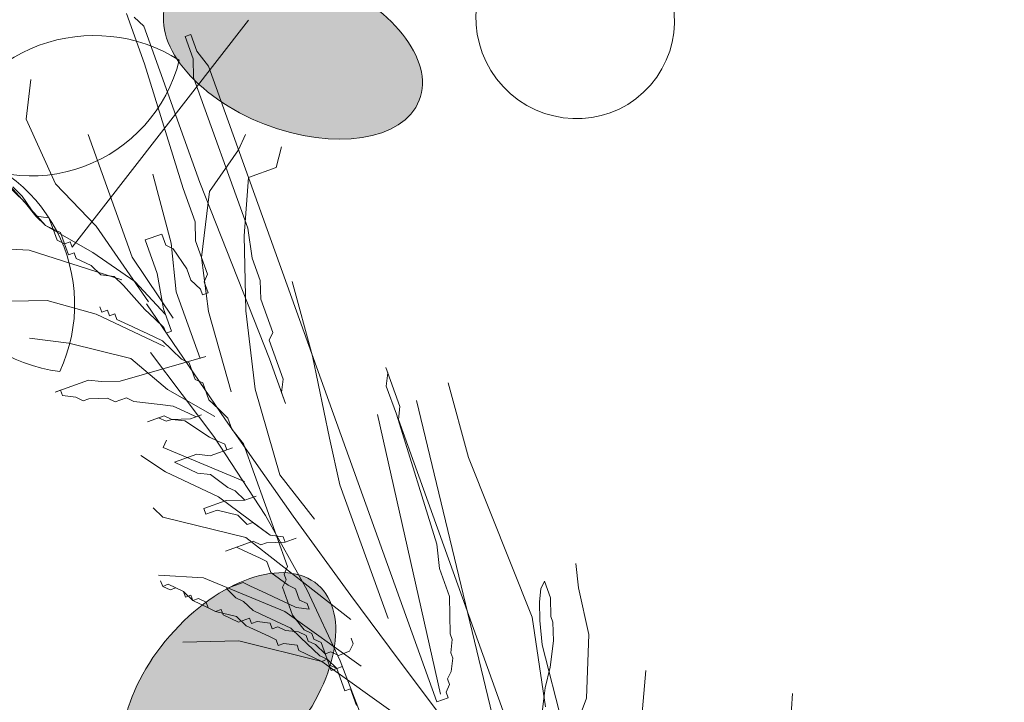
# Model space of a CAD drawing. Units: millimetres. Extents: x 595116 to 630915, y 909473 to 920225.
# Tile 102 of 134: x 629803.095 to 629807.854, y 919177.721 to 919181.018. Entities that reach past the tile are written whole.
import ezdxf

# ---------------------------------------------------------------- set-up
doc = ezdxf.new("R2010")
doc.units = ezdxf.units.MM
doc.layers.add('L-PLNT', color=85, linetype='Continuous', lineweight=13)

# ---------------------------------------------------------------- blocks, each defined once
blk = doc.blocks.new('A$C4FB75ABC')
for p, q in [((2.1583, 4.4143), (2.3852, 4.7066)), ((2.2283, 4.715), (2.2515, 4.6504)), ((2.2504, 4.6987), (2.238, 4.7104)), ((2.3227, 4.4977), (2.2504, 4.6987)), ((2.3109, 4.688), (2.3037, 4.6854)), ((2.3037, 4.6854), (2.314, 4.6567)), ((2.3186, 4.6665), (2.3109, 4.688)), ((2.3336, 4.6475), (2.3186, 4.6665)), ((2.314, 4.6567), (2.3146, 4.6326)), ((2.2515, 4.6504), (2.3011, 4.49)), ((2.6279, 3.8295), (2.3336, 4.6475)), ((2.0989, 4.5793), (2.1049, 4.6301)), ((2.3146, 4.6326), (2.3843, 4.4389)), ((2.137, 4.4958), (2.0989, 4.5793)), ((2.1238, 4.4424), (2.0025, 4.577)), ((2.197, 4.5092), (2.1789, 4.5595)), ((2.3723, 4.5399), (2.3815, 4.5594)), ((2.335, 4.486), (2.3723, 4.5399)), ((2.4211, 4.5169), (2.4277, 4.5436)), ((2.3852, 4.504), (2.4211, 4.5169)), ((2.2357, 4.4016), (2.197, 4.5092)), ((2.2859, 4.4197), (2.2621, 4.5084)), ((2.3797, 4.4291), (2.3852, 4.504)), ((2.0719, 4.4967), (2.0966, 4.4731)), ((2.094, 4.4803), (2.0817, 4.4921)), ((2.189, 4.4415), (2.137, 4.4958)), ((2.3011, 4.49), (2.3166, 4.4469)), ((2.4125, 4.2707), (2.3227, 4.4977)), ((2.1115, 4.4542), (2.094, 4.4803)), ((2.325, 4.4013), (2.335, 4.486)), ((2.0966, 4.4731), (2.1115, 4.4542)), ((2.1238, 4.4424), (2.1115, 4.4542)), ((2.1115, 4.4542), (2.1284, 4.4522)), ((2.1284, 4.4522), (2.1336, 4.4378)), ((2.1336, 4.4378), (2.1238, 4.4424)), ((2.185, 4.4077), (2.1238, 4.4424)), ((2.1388, 4.4235), (2.1336, 4.4378)), ((2.1336, 4.4378), (2.1434, 4.4332)), ((2.2564, 4.3442), (2.189, 4.4415)), ((2.3166, 4.4469), (2.3172, 4.4228)), ((2.3843, 4.4389), (2.3901, 4.4004)), ((2.1434, 4.4332), (2.1485, 4.4189)), ((2.2736, 4.4314), (2.2521, 4.4237)), ((2.2788, 4.4171), (2.2736, 4.4314)), ((2.382, 4.3327), (2.3797, 4.4291)), ((2.1029, 4.4105), (2.0449, 4.414)), ((2.1485, 4.4189), (2.1388, 4.4235)), ((2.1485, 4.4189), (2.1557, 4.4214)), ((2.1537, 4.4045), (2.1485, 4.4189)), ((2.1557, 4.4214), (2.1583, 4.4143)), ((2.2521, 4.4237), (2.2676, 4.3807)), ((2.2885, 4.4125), (2.2788, 4.4171)), ((2.2922, 4.3571), (2.2859, 4.4197)), ((2.306, 4.3864), (2.2885, 4.4125)), ((2.3172, 4.4228), (2.3327, 4.3798)), ((2.222, 4.3723), (2.1029, 4.4105)), ((2.1609, 4.4071), (2.1537, 4.4045)), ((2.1634, 4.3999), (2.1609, 4.4071)), ((2.1829, 4.3907), (2.1634, 4.3999)), ((2.2389, 4.3703), (2.185, 4.4077)), ((2.2882, 4.3232), (2.2357, 4.4016)), ((2.3338, 4.3316), (2.325, 4.4013)), ((2.3901, 4.4004), (2.4004, 4.3717)), ((2.1953, 4.379), (2.1829, 4.3907)), ((2.2122, 4.3769), (2.1953, 4.379)), ((2.2245, 4.3652), (2.2122, 4.3769)), ((2.2676, 4.3807), (2.2759, 4.335)), ((2.3112, 4.372), (2.306, 4.3864)), ((2.3327, 4.3798), (2.3281, 4.37)), ((2.2518, 4.3344), (2.2245, 4.3652)), ((2.2785, 4.3278), (2.2389, 4.3703)), ((2.3235, 4.3603), (2.3112, 4.372)), ((2.3281, 4.37), (2.3333, 4.3557)), ((2.4004, 4.3717), (2.401, 4.3476)), ((2.4678, 4.2744), (2.4414, 4.3703)), ((2.3232, 4.271), (2.2922, 4.3571)), ((2.3261, 4.3531), (2.3235, 4.3603)), ((2.3333, 4.3557), (2.3261, 4.3531)), ((2.1261, 4.346), (2.0779, 4.3448)), ((2.1893, 4.3282), (2.1261, 4.346)), ((2.1938, 4.3379), (2.1964, 4.3307)), ((2.2538, 4.3417), (2.3557, 4.1924)), ((2.401, 4.3476), (2.4165, 4.3046)), ((2.277, 4.2868), (2.1893, 4.3282)), ((2.1964, 4.3307), (2.2036, 4.3333)), ((2.2036, 4.3333), (2.2062, 4.3261)), ((2.2062, 4.3261), (2.2134, 4.3287)), ((2.2134, 4.3287), (2.2159, 4.3215)), ((2.2641, 4.3227), (2.2518, 4.3344)), ((2.2759, 4.335), (2.2862, 4.3063)), ((2.3628, 4.2285), (2.3338, 4.3316)), ((2.3941, 4.2317), (2.382, 4.3327)), ((2.2159, 4.3215), (2.2354, 4.3124)), ((2.2354, 4.3124), (2.2452, 4.3078)), ((2.2765, 4.3109), (2.2641, 4.3227)), ((2.2791, 4.3037), (2.2765, 4.3109)), ((2.2452, 4.3078), (2.255, 4.3032)), ((2.255, 4.3032), (2.2745, 4.294)), ((2.2862, 4.3063), (2.2791, 4.3037)), ((2.4165, 4.3046), (2.4119, 4.2948)), ((2.154, 4.2911), (2.1032, 4.2972)), ((2.234, 4.2713), (2.154, 4.2911)), ((2.2745, 4.294), (2.2868, 4.2822)), ((2.4119, 4.2948), (2.43, 4.2446)), ((2.2202, 4.242), (2.3304, 4.2736)), ((2.3407, 4.1707), (2.2593, 4.2788)), ((2.2868, 4.2822), (2.2991, 4.2704)), ((2.4896, 4.1688), (2.4678, 4.2744)), ((2.2808, 4.2314), (2.234, 4.2713)), ((2.2991, 4.2704), (2.3089, 4.2658)), ((2.3089, 4.2658), (2.3166, 4.2443)), ((2.4331, 4.2133), (2.4125, 4.2707)), ((2.5803, 4.2095), (2.5622, 4.2597)), ((2.5622, 4.2597), (2.5648, 4.2526)), ((2.5648, 4.2526), (2.5628, 4.2356)), ((2.1362, 4.228), (2.1792, 4.2435)), ((2.1792, 4.2435), (2.1961, 4.2415)), ((2.1961, 4.2415), (2.2202, 4.242)), ((2.3166, 4.2443), (2.3264, 4.2397)), ((2.3264, 4.2397), (2.3341, 4.2182)), ((2.43, 4.2446), (2.4279, 4.2276)), ((2.5628, 4.2356), (2.5757, 4.1997)), ((2.6686, 4.144), (2.6423, 4.2399)), ((2.1434, 4.2306), (2.1362, 4.228)), ((2.1459, 4.2234), (2.1434, 4.2306)), ((2.1629, 4.2214), (2.1459, 4.2234)), ((2.3419, 4.1967), (2.2808, 4.2314)), ((2.4257, 4.1214), (2.3941, 4.2317)), ((2.4279, 4.2276), (2.4331, 4.2133)), ((2.1726, 4.2168), (2.1629, 4.2214)), ((2.1798, 4.2194), (2.1726, 4.2168)), ((2.2039, 4.22), (2.1798, 4.2194)), ((2.2136, 4.2154), (2.2039, 4.22)), ((2.228, 4.2205), (2.2136, 4.2154)), ((2.2377, 4.2159), (2.228, 4.2205)), ((2.2716, 4.2119), (2.2377, 4.2159)), ((2.2885, 4.2099), (2.2716, 4.2119)), ((2.308, 4.2007), (2.2885, 4.2099)), ((2.3341, 4.2182), (2.3465, 4.2064)), ((2.5783, 4.1926), (2.5803, 4.2095)), ((2.7169, 3.7399), (2.6018, 4.2172)), ((2.2552, 4.1898), (2.2768, 4.1975)), ((2.2768, 4.1975), (2.2865, 4.1929)), ((2.3178, 4.1961), (2.308, 4.2007)), ((2.3106, 4.1935), (2.325, 4.1987)), ((2.325, 4.1987), (2.3178, 4.1961)), ((2.3465, 4.2064), (2.3588, 4.1946)), ((2.6325, 3.8393), (2.5516, 4.1992)), ((2.5757, 4.1997), (2.6279, 4.0321)), ((2.2696, 4.195), (2.2552, 4.1898)), ((2.2793, 4.1904), (2.2696, 4.195)), ((2.2865, 4.1929), (2.2793, 4.1904)), ((2.2865, 4.1929), (2.3106, 4.1935)), ((2.3034, 4.1909), (2.2865, 4.1929)), ((2.3353, 4.17), (2.3034, 4.1909)), ((2.3557, 4.1924), (2.443, 4.0685)), ((2.3588, 4.1946), (2.364, 4.1803)), ((2.8029, 3.5683), (2.5783, 4.1926)), ((2.364, 4.1803), (2.3789, 4.1614)), ((2.2753, 4.1565), (2.2799, 4.1663)), ((2.345, 4.1654), (2.3353, 4.17)), ((2.4072, 4.0691), (2.3407, 4.1707)), ((2.3548, 4.1608), (2.345, 4.1654)), ((2.3574, 4.1536), (2.3548, 4.1608)), ((2.3789, 4.1614), (2.4357, 4.0035)), ((2.5031, 4.1088), (2.4896, 4.1688)), ((2.2785, 4.1252), (2.2466, 4.1462)), ((2.38, 4.1131), (2.2753, 4.1565)), ((2.2902, 4.1376), (2.3189, 4.1479)), ((2.3189, 4.1479), (2.3359, 4.1459)), ((2.3359, 4.1459), (2.3645, 4.1562)), ((2.3645, 4.1562), (2.3574, 4.1536)), ((2.3, 4.133), (2.2902, 4.1376)), ((2.7507, 3.9385), (2.6686, 4.144)), ((2.3468, 4.0931), (2.2785, 4.1252)), ((2.3098, 4.1284), (2.3, 4.133)), ((2.3195, 4.1238), (2.3098, 4.1284)), ((2.3364, 4.1218), (2.3195, 4.1238)), ((2.3585, 4.1054), (2.3364, 4.1218)), ((2.4704, 4.0646), (2.4257, 4.1214)), ((2.5651, 3.9366), (2.5031, 4.1088)), ((2.3683, 4.1008), (2.3585, 4.1054)), ((2.3806, 4.089), (2.3683, 4.1008)), ((2.3278, 4.0781), (2.3565, 4.0885)), ((2.413, 4.044), (2.3468, 4.0931)), ((2.3565, 4.0885), (2.3806, 4.089)), ((2.3806, 4.089), (2.395, 4.0942)), ((2.395, 4.0942), (2.3806, 4.089)), ((2.275, 4.0672), (2.2627, 4.079)), ((2.3304, 4.071), (2.3278, 4.0781)), ((2.3448, 4.0761), (2.3304, 4.071)), ((2.3714, 4.0695), (2.3448, 4.0761)), ((2.3818, 4.0408), (2.275, 4.0672)), ((2.3838, 4.0577), (2.3714, 4.0695)), ((2.3909, 4.0603), (2.3838, 4.0577)), ((2.413, 4.044), (2.3909, 4.0603)), ((2.4608, 3.9732), (2.4072, 4.0691)), ((2.443, 4.0685), (2.5171, 3.9664)), ((2.3557, 4.0233), (2.3915, 4.0362)), ((2.5169, 3.9354), (2.3818, 4.0408)), ((2.3915, 4.0362), (2.4013, 4.0316)), ((2.4013, 4.0316), (2.4084, 4.0342)), ((2.4084, 4.0342), (2.4325, 4.0348)), ((2.43, 4.0419), (2.413, 4.044)), ((2.4325, 4.0348), (2.43, 4.0419)), ((2.4325, 4.0348), (2.4469, 4.0399)), ((2.4469, 4.0399), (2.4325, 4.0348)), ((2.6279, 4.0321), (2.6311, 4.0008)), ((2.37, 4.0285), (2.3557, 4.0233)), ((2.3798, 4.0239), (2.37, 4.0285)), ((2.3993, 4.0147), (2.3798, 4.0239)), ((2.409, 4.0101), (2.3993, 4.0147)), ((2.4142, 3.9957), (2.409, 4.0101)), ((2.8101, 3.9761), (2.8069, 4.0074)), ((2.4363, 3.9794), (2.4142, 3.9957)), ((2.4357, 4.0035), (2.4311, 3.9937)), ((2.6311, 4.0008), (2.644, 3.965)), ((2.3275, 3.9889), (2.2696, 3.9923)), ((2.2748, 3.978), (2.2722, 3.9852)), ((2.2722, 3.9852), (2.2748, 3.978)), ((2.4323, 3.9455), (2.3275, 3.9889)), ((2.3568, 3.9751), (2.3783, 3.9828)), ((2.3783, 3.9828), (2.3881, 3.9782)), ((2.4337, 3.9866), (2.4291, 3.9768)), ((2.4311, 3.9937), (2.4337, 3.9866)), ((2.7665, 3.9847), (2.7619, 3.975)), ((2.7742, 3.9632), (2.7665, 3.9847)), ((2.2748, 3.978), (2.2819, 3.9806)), ((2.2845, 3.9734), (2.2748, 3.978)), ((2.2819, 3.9806), (2.2917, 3.976)), ((2.2917, 3.976), (2.2845, 3.9734)), ((2.3014, 3.9714), (2.2917, 3.976)), ((2.2917, 3.976), (2.3014, 3.9714)), ((2.304, 3.9642), (2.3014, 3.9714)), ((2.3014, 3.9714), (2.3138, 3.9596)), ((2.3691, 3.9633), (2.3568, 3.9751)), ((2.3881, 3.9782), (2.4076, 3.9691)), ((2.4076, 3.9691), (2.4173, 3.9645)), ((2.4291, 3.9768), (2.442, 3.9409)), ((2.446, 3.9748), (2.4363, 3.9794)), ((2.4512, 3.9604), (2.446, 3.9748)), ((2.5035, 3.8821), (2.4608, 3.9732)), ((2.7619, 3.975), (2.7599, 3.958)), ((2.8236, 3.9161), (2.8101, 3.9761)), ((2.3112, 3.9668), (2.304, 3.9642)), ((2.3138, 3.9596), (2.3112, 3.9668)), ((2.3209, 3.9622), (2.3138, 3.9596)), ((2.3138, 3.9596), (2.3235, 3.955)), ((2.3307, 3.9576), (2.3209, 3.9622)), ((2.3333, 3.9504), (2.3307, 3.9576)), ((2.3789, 3.9587), (2.3691, 3.9633)), ((2.3912, 3.947), (2.3789, 3.9587)), ((2.4173, 3.9645), (2.4368, 3.9553)), ((2.4609, 3.9558), (2.4512, 3.9604)), ((2.4635, 3.9487), (2.4609, 3.9558)), ((2.5171, 3.9664), (2.5794, 3.8826)), ((2.644, 3.965), (2.6451, 3.9167)), ((2.7599, 3.958), (2.7605, 3.9339)), ((2.7748, 3.9391), (2.7742, 3.9632)), ((2.3235, 3.955), (2.3333, 3.9504)), ((2.343, 3.9458), (2.3333, 3.9504)), ((2.3333, 3.9504), (2.343, 3.9458)), ((2.3502, 3.9484), (2.343, 3.9458)), ((2.343, 3.9458), (2.3697, 3.9392)), ((2.3528, 3.9412), (2.3502, 3.9484)), ((2.401, 3.9424), (2.3912, 3.947)), ((2.5304, 3.8755), (2.4323, 3.9455)), ((2.4368, 3.9553), (2.4466, 3.9507)), ((2.4466, 3.9507), (2.4635, 3.9487)), ((2.3723, 3.932), (2.3528, 3.9412)), ((2.3697, 3.9392), (2.3821, 3.9274)), ((2.3866, 3.9372), (2.3723, 3.932)), ((2.3892, 3.93), (2.3866, 3.9372)), ((2.3964, 3.9326), (2.3892, 3.93)), ((2.4133, 3.9306), (2.3964, 3.9326)), ((2.44, 3.924), (2.401, 3.9424)), ((2.4159, 3.9234), (2.4133, 3.9306)), ((2.442, 3.9409), (2.4569, 3.922)), ((2.7679, 3.8231), (2.7507, 3.9385)), ((2.7605, 3.9339), (2.7636, 3.9026)), ((2.7774, 3.9319), (2.7748, 3.9391)), ((2.778, 3.9078), (2.7774, 3.9319)), ((2.3821, 3.9274), (2.3918, 3.9228)), ((2.3918, 3.9228), (2.4113, 3.9137)), ((2.4231, 3.926), (2.4159, 3.9234)), ((2.4328, 3.9214), (2.4231, 3.926)), ((2.4498, 3.9194), (2.4328, 3.9214)), ((2.4523, 3.9122), (2.44, 3.924)), ((2.4595, 3.9148), (2.4498, 3.9194)), ((2.4569, 3.922), (2.4667, 3.9174)), ((2.3729, 3.9079), (2.3006, 3.9062)), ((2.4796, 3.8815), (2.3729, 3.9079)), ((2.4113, 3.9137), (2.4211, 3.9091)), ((2.4211, 3.9091), (2.4237, 3.9019)), ((2.477, 3.8887), (2.4523, 3.9122)), ((2.4621, 3.9076), (2.4595, 3.9148)), ((2.4718, 3.903), (2.4621, 3.9076)), ((2.4667, 3.9174), (2.4693, 3.9102)), ((2.4693, 3.9102), (2.479, 3.9056)), ((2.479, 3.9056), (2.4868, 3.8841)), ((2.5175, 3.9113), (2.52, 3.9042)), ((2.6451, 3.9167), (2.6477, 3.9096)), ((2.6477, 3.9096), (2.6457, 3.8926)), ((2.7739, 3.8739), (2.778, 3.9078)), ((2.8207, 3.834), (2.8236, 3.9161)), ((2.4237, 3.9019), (2.4308, 3.9045)), ((2.4308, 3.9045), (2.4478, 3.9025)), ((2.4478, 3.9025), (2.4503, 3.8953)), ((2.4503, 3.8953), (2.4698, 3.8861)), ((2.4842, 3.8913), (2.4718, 3.903)), ((2.4914, 3.8938), (2.4842, 3.8913)), ((2.5011, 3.8892), (2.4914, 3.8938)), ((2.5155, 3.8944), (2.5011, 3.8892)), ((2.52, 3.9042), (2.5155, 3.8944)), ((2.6457, 3.8926), (2.6483, 3.8855)), ((2.7636, 3.9026), (2.8247, 3.6653)), ((2.4698, 3.8861), (2.4796, 3.8815)), ((2.4868, 3.8841), (2.477, 3.8887)), ((2.4796, 3.8815), (2.4868, 3.8841)), ((2.5777, 3.8114), (2.4796, 3.8815)), ((2.4868, 3.8841), (2.4893, 3.8769)), ((2.4919, 3.8697), (2.4868, 3.8841)), ((2.4868, 3.8841), (2.4991, 3.8723)), ((2.5372, 3.7949), (2.5035, 3.8821)), ((2.5794, 3.8826), (2.6314, 3.8136)), ((2.6483, 3.8855), (2.6463, 3.8685)), ((2.4893, 3.8769), (2.4991, 3.8723)), ((2.5063, 3.8749), (2.4919, 3.8697)), ((2.4991, 3.8723), (2.5063, 3.8749)), ((2.4991, 3.8723), (2.5094, 3.8436)), ((2.6463, 3.8685), (2.6417, 3.8588)), ((2.7673, 3.8473), (2.7739, 3.8739)), ((2.8876, 3.7608), (2.897, 3.8696)), ((2.6417, 3.8588), (2.6443, 3.8516)), ((2.5094, 3.8436), (2.5166, 3.8462)), ((2.5166, 3.8462), (2.5244, 3.8247)), ((2.6443, 3.8516), (2.6397, 3.8418)), ((2.6397, 3.8418), (2.6423, 3.8347)), ((2.7653, 3.8303), (2.7673, 3.8473)), ((2.6423, 3.8347), (2.6279, 3.8295)), ((2.7613, 3.7965), (2.7653, 3.8303)), ((2.7957, 3.7683), (2.8207, 3.834)), ((3.0823, 3.7823), (3.0858, 3.8403))]:
    blk.add_line(p, q)
blk = doc.blocks.new('A$C77972600')
h = blk.add_hatch(color=256)
edge = h.paths.add_edge_path()
edge.add_ellipse((4.1652, 1.933), major_axis=(0.1866, 0.0058), ratio=0.578492, start_angle=0, end_angle=360)
edge = h.paths.add_edge_path()
edge.add_ellipse((3.2944, 1.3586), major_axis=(0.1739, -0.0678), ratio=0.578492, start_angle=0, end_angle=360)
edge = h.paths.add_edge_path()
edge.add_ellipse((3.2064, 0.4835), major_axis=(0.1223, 0.141), ratio=0.578492, start_angle=0, end_angle=360)
edge = h.paths.add_edge_path()
edge.add_ellipse((2.6497, 0.127), major_axis=(0.1678, 0.0818), ratio=0.578492, start_angle=0, end_angle=360)
edge = h.paths.add_edge_path()
edge.add_ellipse((1.7252, 3.461), major_axis=(0.1678, 0.0818), ratio=0.578492, start_angle=0, end_angle=360)
edge = h.paths.add_edge_path()
edge.add_ellipse((2.1962, 2.8048), major_axis=(0.1678, 0.0818), ratio=0.578492, start_angle=0, end_angle=360)
edge = h.paths.add_edge_path()
edge.add_ellipse((1.7372, 2.8674), major_axis=(0.1866, 0.0058), ratio=0.578492, start_angle=0, end_angle=360)
edge = h.paths.add_edge_path()
edge.add_ellipse((3.2773, 2.4479), major_axis=(0.1739, -0.0678), ratio=0.578492, start_angle=0, end_angle=360)
edge = h.paths.add_edge_path()
edge.add_ellipse((3.6722, 2.9717), major_axis=(0.1739, -0.0678), ratio=0.578492, start_angle=0, end_angle=360)
edge = h.paths.add_edge_path()
edge.add_ellipse((2.9739, 2.7963), major_axis=(0.1739, -0.0678), ratio=0.578492, start_angle=0, end_angle=360)
edge = h.paths.add_edge_path()
edge.add_ellipse((4.8796, 2.4604), major_axis=(0.1678, 0.0818), ratio=0.578492, start_angle=0, end_angle=360)
edge = h.paths.add_edge_path()
edge.add_ellipse((4.2454, 2.1577), major_axis=(0.1678, 0.0818), ratio=0.578492, start_angle=0, end_angle=360)
edge = h.paths.add_edge_path()
edge.add_ellipse((4.4178, 2.4738), major_axis=(0.1678, 0.0818), ratio=0.578492, start_angle=0, end_angle=360)
edge = h.paths.add_edge_path()
edge.add_ellipse((4.3066, 3.973), major_axis=(0.1866, 0.0058), ratio=0.578492, start_angle=0, end_angle=360)
edge = h.paths.add_edge_path()
edge.add_ellipse((3.0828, 1.7149), major_axis=(0.1223, 0.141), ratio=0.578492, start_angle=0, end_angle=360)
edge = h.paths.add_edge_path()
edge.add_ellipse((4.1152, 4.8113), major_axis=(0.1678, 0.0818), ratio=0.578492, start_angle=0, end_angle=360)
edge = h.paths.add_edge_path()
edge.add_ellipse((4.4995, 4.8518), major_axis=(0.1223, 0.141), ratio=0.578492, start_angle=0, end_angle=360)
edge = h.paths.add_edge_path()
edge.add_ellipse((4.913, 5.2627), major_axis=(0.1678, 0.0818), ratio=0.578492, start_angle=0, end_angle=360)
edge = h.paths.add_edge_path()
edge.add_ellipse((5.0407, 4.562), major_axis=(0.1223, 0.141), ratio=0.578492, start_angle=0, end_angle=360)
edge = h.paths.add_edge_path()
edge.add_ellipse((4.6105, 4.3933), major_axis=(0.1223, 0.141), ratio=0.578492, start_angle=0, end_angle=360)
edge = h.paths.add_edge_path()
edge.add_ellipse((5.7235, 4.0986), major_axis=(0.1866, 0.0058), ratio=0.578492, start_angle=0, end_angle=360)
edge = h.paths.add_edge_path()
edge.add_ellipse((5.9977, 3.3249), major_axis=(0.1739, -0.0678), ratio=0.578492, start_angle=0, end_angle=360)
edge = h.paths.add_edge_path()
edge.add_ellipse((5.6486, 3.2372), major_axis=(0.1739, -0.0678), ratio=0.578492, start_angle=0, end_angle=360)
edge = h.paths.add_edge_path()
edge.add_ellipse((1.5981, 2.014), major_axis=(0.1678, 0.0818), ratio=0.578492, start_angle=0, end_angle=360)
edge = h.paths.add_edge_path()
edge.add_ellipse((2.2453, 5.0931), major_axis=(0.1678, 0.0818), ratio=0.578492, start_angle=0, end_angle=360)
edge = h.paths.add_edge_path()
edge.add_ellipse((2.073, 4.777), major_axis=(0.1678, 0.0818), ratio=0.578492, start_angle=0, end_angle=360)
edge = h.paths.add_edge_path()
edge.add_ellipse((1.2216, 4.5968), major_axis=(0.1866, 0.0058), ratio=0.578492, start_angle=0, end_angle=360)
edge = h.paths.add_edge_path()
edge.add_ellipse((1.6688, 4.0227), major_axis=(0.1866, 0.0058), ratio=0.578492, start_angle=0, end_angle=360)
edge = h.paths.add_edge_path()
edge.add_ellipse((1.253, 4.2244), major_axis=(0.1866, 0.0058), ratio=0.578492, start_angle=0, end_angle=360)
edge = h.paths.add_edge_path()
edge.add_ellipse((2.3257, 4.3332), major_axis=(0.1866, 0.0058), ratio=0.578492, start_angle=0, end_angle=360)
for centre, radius, start, end in [((3.0209, 1.1614), 0.2185, 57.5868, 162.9238), ((2.9338, 1.3974), 0.2106, 234.6671, 345.8435), ((2.9982, 1.1271), 0.2106, 152.1384, 263.3149), ((2.7756, 1.0101), 0.2185, 335.0581, 80.3951)]:
    blk.add_arc(centre, radius, start, end)
blk.add_ellipse((3.6829, 1.4023), major_axis=(-0.0941, 0.1005), ratio=0.985729)
for centre, major_axis in [((3.2944, 1.3586), (-0.1739, 0.0678)), ((3.2064, 0.4835), (-0.1223, -0.141))]:
    blk.add_ellipse(centre, major_axis=major_axis, ratio=0.578492, start_param=3.141593, end_param=9.424778)

msp = doc.modelspace()

# ---------------------------------------------------------------- block references
at = {"layer": 'L-PLNT'}
for name, p, xscale, yscale, zscale in [('A$C77972600', (629792.8437, 919176.0945), 3.512546757812034, 3.512546757812034, 3.512546757812034), ('A$C4FB75ABC', (629795.2477, 919163.3497), 3.753413438031968, 3.753413438031968, 3.753413438031968)]:
    msp.add_blockref(name, p, dxfattribs=dict(at, xscale=xscale, yscale=yscale, zscale=zscale))

doc.saveas('drawing.dxf')
